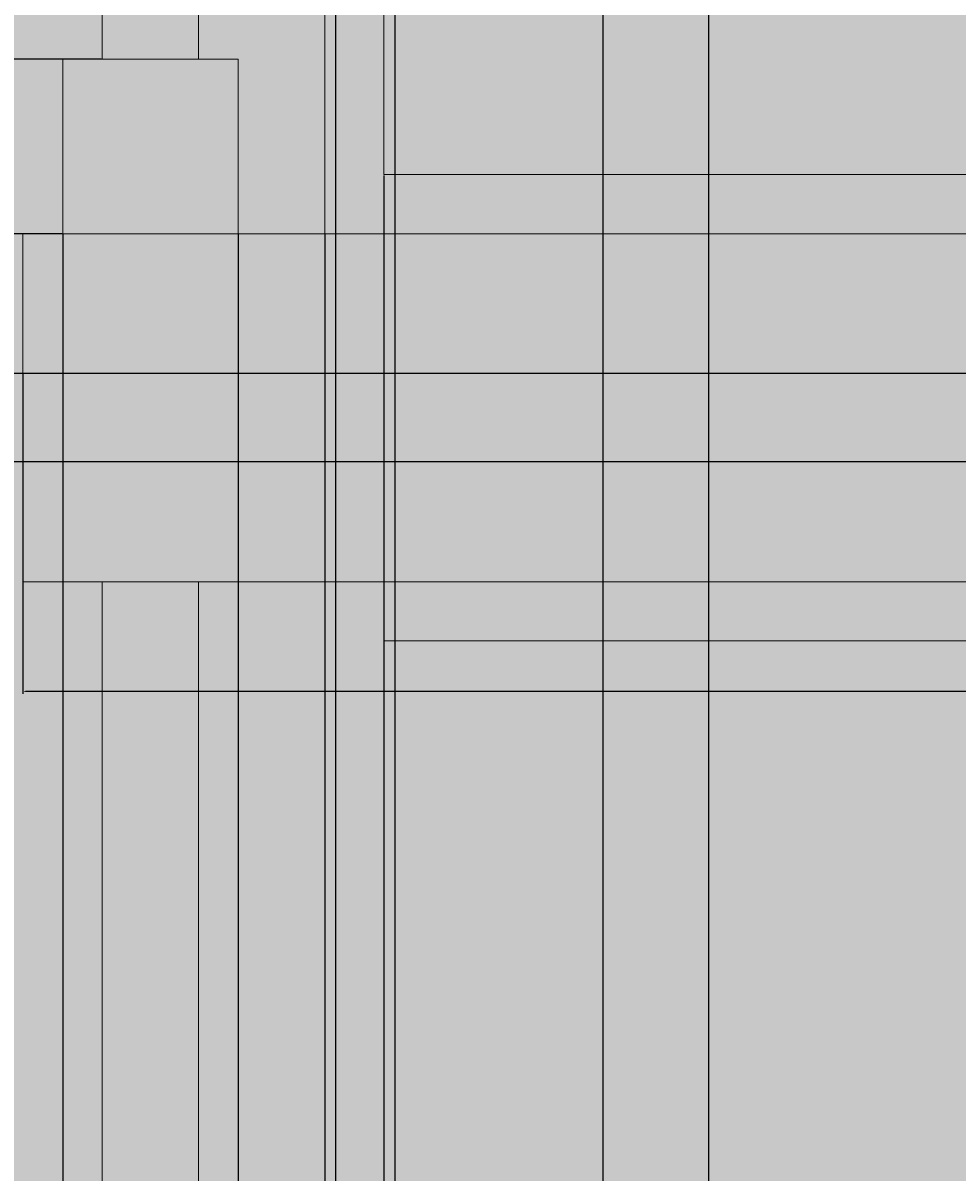
# Model space of a CAD drawing. Units: inches. Extents: x 3024 to 4744, y 1110 to 2100.
# Tile 20 of 29: x 3149 to 3212, y 1731 to 1809. Entities that reach past the tile are written whole.
import ezdxf

# ---------------------------------------------------------------- set-up
doc = ezdxf.new("R2010")
doc.units = ezdxf.units.IN
for name, color, linetype, lineweight in [('A-ANNO-DIMS', 2, 'Continuous', 18), ('A-ELEV', 7, 'Continuous', 25), ('A-ELEV-PATT', 252, 'Continuous', 13), ('A-GLAZ', 4, 'Continuous', 18)]:
    doc.layers.add(name, color=color, linetype=linetype, lineweight=lineweight)
doc.styles.get("Standard").update_dxf_attribs({"font": 'arial.ttf'})
doc.dimstyles.get("Standard").update_dxf_attribs({"dimtxt": 0.18, "dimasz": 0.18, "dimexe": 0.18, "dimexo": 0.0625, "dimgap": 0.09, "dimtad": 0, "dimtih": 1, "dimtoh": 1, "dimdec": 1, "dimzin": 0, "dimdsep": 46, "dimlunit": 3, "dimtxsty": 'Standard', "dimcen": 0.09, "dimadec": 0, "dimazin": 0, "dimtfac": 1, "dimtdec": 1, "dimtofl": 0, "dimtmove": 0, "dimatfit": 3, "dimfxl": 1, "dimtolj": 1, "dimtzin": 0, "dimarcsym": 0})

# ---------------------------------------------------------------- blocks, each defined once
blk = doc.blocks.new('WIN-BALCONY-A')
for p, q in [((3169.396, 1897.488), (3148.969, 1897.488)), ((3169.396, 1897.488), (3148.969, 1897.488)), ((3169.396, 1897.488), (3292.605, 1897.488)), ((3169.396, 1897.488), (3292.605, 1897.488)), ((3169.396, 1795.043), (3148.969, 1795.043)), ((3169.396, 1795.043), (3148.969, 1795.043)), ((3169.396, 1795.043), (3292.605, 1795.043)), ((3169.396, 1795.043), (3292.605, 1795.043))]:
    blk.add_line(p, q)
for points in [[(3148.969, 1897.488), (3148.969, 1905.611), (3292.605, 1905.611), (3292.605, 1897.488)], [(3148.969, 1897.488), (3148.969, 1905.611), (3292.605, 1905.611), (3292.605, 1897.488)], [(3292.605, 1795.043), (3292.605, 1785.611), (3148.969, 1785.611), (3148.969, 1795.043)], [(3292.605, 1795.043), (3292.605, 1785.611), (3148.969, 1785.611), (3148.969, 1795.043)]]:
    blk.add_lwpolyline(points)
for points in [[(3154.329, 1806.867), (3160.859, 1806.867), (3160.859, 1897.488), (3154.329, 1897.488)], [(3154.329, 1806.867), (3160.859, 1806.867), (3160.859, 1897.488), (3154.329, 1897.488)], [(3272.178, 1795.043), (3169.396, 1795.043), (3169.396, 1897.488), (3272.178, 1897.488)], [(3272.178, 1795.043), (3169.396, 1795.043), (3169.396, 1897.488), (3272.178, 1897.488)], [(3268.178, 1799.043), (3173.396, 1799.043), (3173.396, 1893.488), (3268.178, 1893.488)], [(3268.178, 1799.043), (3173.396, 1799.043), (3173.396, 1893.488), (3268.178, 1893.488)], [(3163.527, 1795.043), (3151.66, 1795.043), (3151.66, 1806.867), (3163.527, 1806.867)], [(3163.527, 1795.043), (3151.66, 1795.043), (3151.66, 1806.867), (3163.527, 1806.867)]]:
    blk.add_lwpolyline(points, close=True)
blk = doc.blocks.new('*D6')
at = {"layer": 'A-ANNO-DIMS', "color": 0, "lineweight": -2, "transparency": 16777216}
for p, q in [((3148.969, 1785.549), (3148.969, 1763.886)), ((3292.605, 1785.549), (3292.605, 1763.886)), ((3149.149, 1764.066), (3218.852, 1764.066)), ((3292.425, 1764.066), (3222.723, 1764.066))]:
    blk.add_line(p, q, dxfattribs=at)
at = {"layer": 'A-ANNO-DIMS', "color": 0, "transparency": 16777216}
for points in [[(3149.149, 1764.096), (3149.149, 1764.036), (3148.969, 1764.066)], [(3292.425, 1764.096), (3292.425, 1764.036), (3292.605, 1764.066)]]:
    blk.add_solid(points, dxfattribs=at)
at = {"layer": 'Defpoints', "color": 0, "transparency": 16777216}
for p in [(3148.969, 1785.611), (3292.605, 1785.611), (3292.605, 1764.066)]:
    blk.add_point(p, dxfattribs=at)
at = {"layer": 'A-ANNO-DIMS', "color": 0, "transparency": 16777216, "insert": (3220.787, 1764.066), "char_height": 0.18, "attachment_point": 5}
blk.add_mtext('\\A1;BALCONY WINDOW A 144 TYP.', dxfattribs=at)
blk = doc.blocks.new('*D64')
at = {"layer": 'A-ANNO-DIMS', "color": 0, "lineweight": -2, "transparency": 16777216}
for p, q in [((3069.794, 1241.497), (3069.794, 2100.438)), ((3741.151, 1241.497), (3741.151, 2100.438)), ((3069.974, 2100.258), (3405.078, 2100.258)), ((3740.971, 2100.258), (3405.866, 2100.258))]:
    blk.add_line(p, q, dxfattribs=at)
at = {"layer": 'A-ANNO-DIMS', "color": 0, "transparency": 16777216}
for points in [[(3069.974, 2100.288), (3069.974, 2100.228), (3069.794, 2100.258)], [(3740.971, 2100.288), (3740.971, 2100.228), (3741.151, 2100.258)]]:
    blk.add_solid(points, dxfattribs=at)
at = {"layer": 'Defpoints', "color": 0, "transparency": 16777216}
for p in [(3741.151, 2100.258), (3069.794, 1241.434), (3741.151, 1241.434)]:
    blk.add_point(p, dxfattribs=at)
at = {"layer": 'A-ANNO-DIMS', "color": 0, "transparency": 16777216, "insert": (3405.472, 2100.258), "char_height": 0.18, "attachment_point": 5}
blk.add_mtext('\\A1;671.4', dxfattribs=at)
blk = doc.blocks.new('*D89')
at = {"layer": 'A-ANNO-DIMS', "color": 0, "lineweight": -2, "transparency": 16777216}
for p, q in [((3151.66, 1794.981), (3151.66, 1109.931)), ((3163.527, 1794.981), (3163.527, 1109.931)), ((3151.84, 1110.111), (3157.139, 1110.111)), ((3163.347, 1110.111), (3158.049, 1110.111))]:
    blk.add_line(p, q, dxfattribs=at)
at = {"layer": 'A-ANNO-DIMS', "color": 0, "transparency": 16777216}
for points in [[(3151.84, 1110.141), (3151.84, 1110.081), (3151.66, 1110.111)], [(3163.347, 1110.141), (3163.347, 1110.081), (3163.527, 1110.111)]]:
    blk.add_solid(points, dxfattribs=at)
at = {"layer": 'Defpoints', "color": 0, "transparency": 16777216}
for p in [(3151.66, 1795.043), (3163.527, 1795.043), (3163.527, 1110.111)]:
    blk.add_point(p, dxfattribs=at)
at = {"layer": 'A-ANNO-DIMS', "color": 0, "transparency": 16777216, "insert": (3157.594, 1110.111), "char_height": 0.18, "attachment_point": 5}
blk.add_mtext('\\A1;11.866', dxfattribs=at)
blk = doc.blocks.new('*D90')
at = {"layer": 'A-ANNO-DIMS', "color": 0, "lineweight": -2, "transparency": 16777216}
for p, q in [((3173.396, 1798.981), (3173.396, 1109.931)), ((3169.396, 1794.981), (3169.396, 1109.931)), ((3169.576, 1110.111), (3171.069, 1110.111)), ((3173.216, 1110.111), (3171.723, 1110.111))]:
    blk.add_line(p, q, dxfattribs=at)
at = {"layer": 'A-ANNO-DIMS', "color": 0, "transparency": 16777216}
for points in [[(3169.576, 1110.141), (3169.576, 1110.081), (3169.396, 1110.111)], [(3173.216, 1110.141), (3173.216, 1110.081), (3173.396, 1110.111)]]:
    blk.add_solid(points, dxfattribs=at)
at = {"layer": 'Defpoints', "color": 0, "transparency": 16777216}
for p in [(3173.396, 1799.043), (3169.396, 1795.043), (3173.396, 1110.111)]:
    blk.add_point(p, dxfattribs=at)
at = {"layer": 'A-ANNO-DIMS', "color": 0, "transparency": 16777216, "insert": (3171.396, 1110.111), "char_height": 0.18, "attachment_point": 5}
blk.add_mtext('\\A1;4.00', dxfattribs=at)
blk = doc.blocks.new('*D91')
at = {"layer": 'A-ANNO-DIMS', "color": 0, "lineweight": -2, "transparency": 16777216}
for p, q in [((3173.396, 1798.981), (3173.396, 1109.931)), ((3220.05, 1798.981), (3220.05, 1109.931)), ((3173.576, 1110.111), (3196.325, 1110.111)), ((3219.87, 1110.111), (3197.121, 1110.111))]:
    blk.add_line(p, q, dxfattribs=at)
at = {"layer": 'A-ANNO-DIMS', "color": 0, "transparency": 16777216}
for points in [[(3173.576, 1110.141), (3173.576, 1110.081), (3173.396, 1110.111)], [(3219.87, 1110.141), (3219.87, 1110.081), (3220.05, 1110.111)]]:
    blk.add_solid(points, dxfattribs=at)
at = {"layer": 'Defpoints', "color": 0, "transparency": 16777216}
for p in [(3173.396, 1799.043), (3220.05, 1799.043), (3220.05, 1110.111)]:
    blk.add_point(p, dxfattribs=at)
at = {"layer": 'A-ANNO-DIMS', "color": 0, "transparency": 16777216, "insert": (3196.723, 1110.111), "char_height": 0.18, "attachment_point": 5}
blk.add_mtext('\\A1;46.65', dxfattribs=at)
blk = doc.blocks.new('*D97')
at = {"layer": 'A-ANNO-DIMS', "color": 0, "lineweight": -2, "transparency": 16777216}
for p, q in [((3151.598, 1806.867), (3024.114, 1806.867)), ((3024.294, 1806.687), (3024.294, 1801.137)), ((3024.294, 1795.223), (3024.294, 1800.773)), ((3151.598, 1795.043), (3024.114, 1795.043))]:
    blk.add_line(p, q, dxfattribs=at)
at = {"layer": 'A-ANNO-DIMS', "color": 0, "transparency": 16777216}
for points in [[(3024.264, 1806.687), (3024.324, 1806.687), (3024.294, 1806.867)], [(3024.264, 1795.223), (3024.324, 1795.223), (3024.294, 1795.043)]]:
    blk.add_solid(points, dxfattribs=at)
at = {"layer": 'Defpoints', "color": 0, "transparency": 16777216}
for p in [(3024.294, 1806.867), (3151.66, 1806.867), (3151.66, 1795.043)]:
    blk.add_point(p, dxfattribs=at)
at = {"layer": 'A-ANNO-DIMS', "color": 0, "transparency": 16777216, "insert": (3024.294, 1800.955), "char_height": 0.18, "attachment_point": 5}
blk.add_mtext('\\A1;11.824', dxfattribs=at)
blk = doc.blocks.new('*D98')
at = {"layer": 'A-ANNO-DIMS', "color": 0, "lineweight": -2, "transparency": 16777216}
for p, q in [((3154.266, 1897.488), (3024.114, 1897.488)), ((3024.294, 1897.308), (3024.294, 1852.36)), ((3024.294, 1807.047), (3024.294, 1851.996)), ((3154.266, 1806.867), (3024.114, 1806.867))]:
    blk.add_line(p, q, dxfattribs=at)
at = {"layer": 'A-ANNO-DIMS', "color": 0, "transparency": 16777216}
for points in [[(3024.264, 1897.308), (3024.324, 1897.308), (3024.294, 1897.488)], [(3024.264, 1807.047), (3024.324, 1807.047), (3024.294, 1806.867)]]:
    blk.add_solid(points, dxfattribs=at)
at = {"layer": 'Defpoints', "color": 0, "transparency": 16777216}
for p in [(3024.294, 1897.488), (3154.329, 1897.488), (3154.329, 1806.867)]:
    blk.add_point(p, dxfattribs=at)
at = {"layer": 'A-ANNO-DIMS', "color": 0, "transparency": 16777216, "insert": (3024.294, 1852.178), "char_height": 0.18, "attachment_point": 5}
blk.add_mtext('\\A1;90.62', dxfattribs=at)
blk = doc.blocks.new('*D106')
at = {"layer": 'A-ANNO-DIMS', "color": 0, "lineweight": -2, "transparency": 16777216}
for p, q in [((3170.161, 1275.674), (3170.161, 2100.438)), ((3174.161, 1271.674), (3174.161, 2100.438)), ((3170.341, 2100.258), (3171.834, 2100.258)), ((3173.981, 2100.258), (3172.488, 2100.258))]:
    blk.add_line(p, q, dxfattribs=at)
at = {"layer": 'A-ANNO-DIMS', "color": 0, "transparency": 16777216}
for points in [[(3170.341, 2100.288), (3170.341, 2100.228), (3170.161, 2100.258)], [(3173.981, 2100.288), (3173.981, 2100.228), (3174.161, 2100.258)]]:
    blk.add_solid(points, dxfattribs=at)
at = {"layer": 'Defpoints', "color": 0, "transparency": 16777216}
for p in [(3174.161, 2100.258), (3170.161, 1275.611), (3174.161, 1271.611)]:
    blk.add_point(p, dxfattribs=at)
at = {"layer": 'A-ANNO-DIMS', "color": 0, "transparency": 16777216, "insert": (3172.161, 2100.258), "char_height": 0.18, "attachment_point": 5}
blk.add_mtext('\\A1;4.00', dxfattribs=at)
blk = doc.blocks.new('*D107')
at = {"layer": 'A-ANNO-DIMS', "color": 0, "lineweight": -2, "transparency": 16777216}
for p, q in [((3174.161, 1271.674), (3174.161, 2100.438)), ((3270.388, 1271.674), (3270.388, 2100.438)), ((3174.341, 2100.258), (3221.881, 2100.258)), ((3270.208, 2100.258), (3222.668, 2100.258))]:
    blk.add_line(p, q, dxfattribs=at)
at = {"layer": 'A-ANNO-DIMS', "color": 0, "transparency": 16777216}
for points in [[(3174.341, 2100.288), (3174.341, 2100.228), (3174.161, 2100.258)], [(3270.208, 2100.288), (3270.208, 2100.228), (3270.388, 2100.258)]]:
    blk.add_solid(points, dxfattribs=at)
at = {"layer": 'Defpoints', "color": 0, "transparency": 16777216}
for p in [(3270.388, 2100.258), (3174.161, 1271.611), (3270.388, 1271.611)]:
    blk.add_point(p, dxfattribs=at)
at = {"layer": 'A-ANNO-DIMS', "color": 0, "transparency": 16777216, "insert": (3222.274, 2100.258), "char_height": 0.18, "attachment_point": 5}
blk.add_mtext('\\A1;96.23', dxfattribs=at)
blk = doc.blocks.new('*D124')
at = {"layer": 'A-ANNO-DIMS', "color": 0, "lineweight": -2, "transparency": 16777216}
for p, q in [((3174.161, 1271.674), (3174.161, 2100.438)), ((3188.259, 1256.29), (3188.259, 2100.438)), ((3174.341, 2100.258), (3180.754, 2100.258)), ((3188.079, 2100.258), (3181.665, 2100.258))]:
    blk.add_line(p, q, dxfattribs=at)
at = {"layer": 'A-ANNO-DIMS', "color": 0, "transparency": 16777216}
for points in [[(3174.341, 2100.288), (3174.341, 2100.228), (3174.161, 2100.258)], [(3188.079, 2100.288), (3188.079, 2100.228), (3188.259, 2100.258)]]:
    blk.add_solid(points, dxfattribs=at)
at = {"layer": 'Defpoints', "color": 0, "transparency": 16777216}
for p in [(3188.259, 2100.258), (3174.161, 1271.611), (3188.259, 1256.228)]:
    blk.add_point(p, dxfattribs=at)
at = {"layer": 'A-ANNO-DIMS', "color": 0, "transparency": 16777216, "insert": (3181.21, 2100.258), "char_height": 0.18, "attachment_point": 5}
blk.add_mtext('\\A1;14.098', dxfattribs=at)
blk = doc.blocks.new('*D125')
at = {"layer": 'A-ANNO-DIMS', "color": 0, "lineweight": -2, "transparency": 16777216}
for p, q in [((3188.259, 1256.29), (3188.259, 2100.438)), ((3195.405, 1256.29), (3195.405, 2100.438)), ((3188.439, 2100.258), (3191.439, 2100.258)), ((3195.225, 2100.258), (3192.225, 2100.258))]:
    blk.add_line(p, q, dxfattribs=at)
at = {"layer": 'A-ANNO-DIMS', "color": 0, "transparency": 16777216}
for points in [[(3188.439, 2100.288), (3188.439, 2100.228), (3188.259, 2100.258)], [(3195.225, 2100.288), (3195.225, 2100.228), (3195.405, 2100.258)]]:
    blk.add_solid(points, dxfattribs=at)
at = {"layer": 'Defpoints', "color": 0, "transparency": 16777216}
for p in [(3195.405, 2100.258), (3188.259, 1256.228), (3195.405, 1256.228)]:
    blk.add_point(p, dxfattribs=at)
at = {"layer": 'A-ANNO-DIMS', "color": 0, "transparency": 16777216, "insert": (3191.832, 2100.258), "char_height": 0.18, "attachment_point": 5}
blk.add_mtext('\\A1;7.147', dxfattribs=at)

msp = doc.modelspace()

# ---------------------------------------------------------------- hatches: boundary and pattern name
at = {"layer": 'A-ELEV-PATT'}
h = msp.add_hatch(color=256, dxfattribs=at)
h.dxf.hatch_style = 1
h.paths.add_polyline_path([(3491.8271, 2054.7584), (3320.5658, 2054.7584), (3320.5658, 2043.5286), (3491.8271, 2043.5286)])
h.paths.add_polyline_path([(3292.6051, 1905.6112), (3148.9694, 1905.6112), (3148.9694, 1897.4879), (3169.3964, 1897.4879), (3292.6051, 1897.4879)])
h.paths.add_polyline_path([(3292.6051, 1795.0431), (3169.3964, 1795.0431), (3148.9694, 1795.0431), (3148.9694, 1785.6112), (3292.6051, 1785.6112)])
h.paths.add_polyline_path([(3292.6051, 1779.6112), (3148.9694, 1779.6112), (3148.9694, 1771.4879), (3169.3964, 1771.4879), (3292.6051, 1771.4879)])
h.paths.add_polyline_path([(3292.6051, 1669.0431), (3169.3964, 1669.0431), (3148.9694, 1669.0431), (3148.9694, 1659.6112), (3292.6051, 1659.6112)])
h.paths.add_polyline_path([(3292.6051, 1653.6112), (3148.9694, 1653.6112), (3148.9694, 1645.4879), (3169.3964, 1645.4879), (3292.6051, 1645.4879)])
h.paths.add_polyline_path([(3292.6051, 1543.0431), (3169.3964, 1543.0431), (3148.9694, 1543.0431), (3148.9694, 1533.6112), (3292.6051, 1533.6112)])
h.paths.add_polyline_path([(3292.6051, 1527.6112), (3148.9694, 1527.6112), (3148.9694, 1519.4879), (3169.3964, 1519.4879), (3292.6051, 1519.4879)])
h.paths.add_polyline_path([(3292.6051, 1401.6112), (3148.9694, 1401.6112), (3148.9694, 1393.4879), (3169.3964, 1393.4879), (3292.6051, 1393.4879)])
h.paths.add_polyline_path([(3292.6051, 1417.0431), (3169.3964, 1417.0431), (3148.9694, 1417.0431), (3148.9694, 1407.6112), (3292.6051, 1407.6112)])
h.paths.add_polyline_path([(3292.6051, 1291.0431), (3169.3964, 1291.0431), (3148.9694, 1291.0431), (3148.9694, 1281.6112), (3292.6051, 1281.6112)])
h.paths.add_polyline_path([(3654.037, 1165.0431), (3530.8283, 1165.0431), (3510.4013, 1165.0431), (3510.4013, 1155.6112), (3654.037, 1155.6112)])
h.paths.add_polyline_path([(3654.037, 1275.6112), (3510.4013, 1275.6112), (3510.4013, 1267.4879), (3530.8283, 1267.4879), (3654.037, 1267.4879)])
h.paths.add_polyline_path([(3654.037, 1291.0431), (3530.8283, 1291.0431), (3510.4013, 1291.0431), (3510.4013, 1281.6112), (3654.037, 1281.6112)])
h.paths.add_polyline_path([(3654.037, 1417.0431), (3530.8283, 1417.0431), (3510.4013, 1417.0431), (3510.4013, 1407.6112), (3654.037, 1407.6112)])
h.paths.add_polyline_path([(3654.037, 1401.6112), (3510.4013, 1401.6112), (3510.4013, 1393.4879), (3530.8283, 1393.4879), (3654.037, 1393.4879)])
h.paths.add_polyline_path([(3654.037, 1543.0431), (3530.8283, 1543.0431), (3510.4013, 1543.0431), (3510.4013, 1533.6112), (3654.037, 1533.6112)])
h.paths.add_polyline_path([(3654.037, 1527.6112), (3510.4013, 1527.6112), (3510.4013, 1519.4879), (3530.8283, 1519.4879), (3654.037, 1519.4879)])
h.paths.add_polyline_path([(3654.037, 1653.6112), (3510.4013, 1653.6112), (3510.4013, 1645.4879), (3530.8283, 1645.4879), (3654.037, 1645.4879)])
h.paths.add_polyline_path([(3654.037, 1669.0431), (3530.8283, 1669.0431), (3510.4013, 1669.0431), (3510.4013, 1659.6112), (3654.037, 1659.6112)])
h.paths.add_polyline_path([(3654.037, 1779.6112), (3510.4013, 1779.6112), (3510.4013, 1771.4879), (3530.8283, 1771.4879), (3654.037, 1771.4879)])
h.paths.add_polyline_path([(3654.037, 1795.0431), (3530.8283, 1795.0431), (3510.4013, 1795.0431), (3510.4013, 1785.6112), (3654.037, 1785.6112)])
h.paths.add_polyline_path([(3654.037, 1905.6112), (3510.4013, 1905.6112), (3510.4013, 1897.4879), (3530.8283, 1897.4879), (3654.037, 1897.4879)])
h = msp.add_hatch(color=256, dxfattribs=at)
h.dxf.hatch_style = 1
h.paths.add_polyline_path([(3329.7033, 1407.6112), (3105.4722, 1407.6112), (3105.4722, 1401.6112), (3329.7033, 1401.6112)])
h.paths.add_polyline_path([(3329.7033, 1281.6112), (3105.4722, 1281.6112), (3105.4722, 1275.6112), (3112.3838, 1275.6112), (3329.7033, 1275.6112)])
h.paths.add_polyline_path([(3329.7033, 1533.6112), (3105.4722, 1533.6112), (3105.4722, 1527.6112), (3329.7033, 1527.6112)])
h.paths.add_polyline_path([(3329.7033, 1659.6112), (3105.4722, 1659.6112), (3105.4722, 1653.6112), (3329.7033, 1653.6112)])
h.paths.add_polyline_path([(3329.7033, 1785.6112), (3105.4722, 1785.6112), (3105.4722, 1779.6112), (3329.7033, 1779.6112)])
h.paths.add_polyline_path([(3329.7033, 1911.6112), (3105.4722, 1911.6112), (3095.7158, 1911.6112), (3095.7158, 1905.6112), (3329.7033, 1905.6112)])
h.paths.add_polyline_path([(3715.2286, 1911.6112), (3705.4722, 1911.6112), (3705.4722, 1905.6112), (3715.2286, 1905.6112)])
h.paths.add_polyline_path([(3688.5588, 1911.6112), (3481.2411, 1911.6112), (3481.2411, 1905.6112), (3688.5588, 1905.6112)])
h = msp.add_hatch(color=256, dxfattribs=at)
h.dxf.hatch_style = 1
h.paths.add_polyline_path([(3154.3287, 1897.4879), (3148.9694, 1897.4879), (3148.9694, 1905.6112), (3105.4722, 1905.6112), (3105.4722, 1785.6112), (3148.9694, 1785.6112), (3148.9694, 1795.0431), (3151.6604, 1795.0431), (3151.6604, 1806.8674), (3154.3287, 1806.8674)])
h.paths.add_polyline_path([(3329.7033, 1905.6112), (3292.6051, 1905.6112), (3292.6051, 1897.4879), (3287.2458, 1897.4879), (3287.2458, 1806.8674), (3288.3759, 1806.8674), (3288.3759, 1795.0431), (3292.6051, 1795.0431), (3292.6051, 1785.6112), (3329.7033, 1785.6112)])
h.paths.add_polyline_path([(3154.3287, 1771.4879), (3148.9694, 1771.4879), (3148.9694, 1779.6112), (3105.4722, 1779.6112), (3105.4722, 1659.6112), (3148.9694, 1659.6112), (3148.9694, 1669.0431), (3151.6604, 1669.0431), (3151.6604, 1680.8674), (3154.3287, 1680.8674)])
h.paths.add_polyline_path([(3329.7033, 1779.6112), (3292.6051, 1779.6112), (3292.6051, 1771.4879), (3287.2458, 1771.4879), (3287.2458, 1680.8674), (3288.3759, 1680.8674), (3288.3759, 1669.0431), (3292.6051, 1669.0431), (3292.6051, 1659.6112), (3329.7033, 1659.6112)])
h.paths.add_polyline_path([(3154.3287, 1645.4879), (3148.9694, 1645.4879), (3148.9694, 1653.6112), (3105.4722, 1653.6112), (3105.4722, 1533.6112), (3148.9694, 1533.6112), (3148.9694, 1543.0431), (3151.6604, 1543.0431), (3151.6604, 1554.8674), (3154.3287, 1554.8674)])
h.paths.add_polyline_path([(3329.7033, 1653.6112), (3292.6051, 1653.6112), (3292.6051, 1645.4879), (3287.2458, 1645.4879), (3287.2458, 1554.8674), (3288.3759, 1554.8674), (3288.3759, 1543.0431), (3292.6051, 1543.0431), (3292.6051, 1533.6112), (3329.7033, 1533.6112)])
h.paths.add_polyline_path([(3329.7033, 1527.6112), (3292.6051, 1527.6112), (3292.6051, 1519.4879), (3287.2458, 1519.4879), (3287.2458, 1428.8674), (3288.3759, 1428.8674), (3288.3759, 1417.0431), (3292.6051, 1417.0431), (3292.6051, 1407.6112), (3329.7033, 1407.6112)])
h.paths.add_polyline_path([(3329.7033, 1401.6112), (3292.6051, 1401.6112), (3292.6051, 1393.4879), (3287.2458, 1393.4879), (3287.2458, 1302.8674), (3288.3759, 1302.8674), (3288.3759, 1291.0431), (3292.6051, 1291.0431), (3292.6051, 1281.6112), (3329.7033, 1281.6112)])
h.paths.add_polyline_path([(3154.3287, 1393.4879), (3148.9694, 1393.4879), (3148.9694, 1401.6112), (3105.4722, 1401.6112), (3105.4722, 1281.6112), (3148.9694, 1281.6112), (3148.9694, 1291.0431), (3151.6604, 1291.0431), (3151.6604, 1302.8674), (3154.3287, 1302.8674)])
h.paths.add_polyline_path([(3154.3287, 1519.4879), (3148.9694, 1519.4879), (3148.9694, 1527.6112), (3105.4722, 1527.6112), (3105.4722, 1407.6112), (3148.9694, 1407.6112), (3148.9694, 1417.0431), (3151.6604, 1417.0431), (3151.6604, 1428.8674), (3154.3287, 1428.8674)])
h.paths.add_polyline_path([(3515.7606, 1897.4879), (3510.4013, 1897.4879), (3510.4013, 1905.6112), (3481.2411, 1905.6112), (3481.2411, 1785.6112), (3510.4013, 1785.6112), (3510.4013, 1795.0431), (3513.0923, 1795.0431), (3513.0923, 1806.8674), (3515.7606, 1806.8674)])
h.paths.add_polyline_path([(3688.5588, 1905.6112), (3654.037, 1905.6112), (3654.037, 1897.4879), (3648.6777, 1897.4879), (3648.6777, 1806.8674), (3649.8078, 1806.8674), (3649.8078, 1795.0431), (3654.037, 1795.0431), (3654.037, 1785.6112), (3688.5588, 1785.6112)])
h.paths.add_polyline_path([(3515.7606, 1771.4879), (3510.4013, 1771.4879), (3510.4013, 1779.6112), (3481.2411, 1779.6112), (3481.2411, 1659.6112), (3510.4013, 1659.6112), (3510.4013, 1669.0431), (3513.0923, 1669.0431), (3513.0923, 1680.8674), (3515.7606, 1680.8674)])
h.paths.add_polyline_path([(3688.5588, 1779.6112), (3654.037, 1779.6112), (3654.037, 1771.4879), (3648.6777, 1771.4879), (3648.6777, 1680.8674), (3649.8078, 1680.8674), (3649.8078, 1669.0431), (3654.037, 1669.0431), (3654.037, 1659.6112), (3688.5588, 1659.6112)])
h.paths.add_polyline_path([(3515.7606, 1645.4879), (3510.4013, 1645.4879), (3510.4013, 1653.6112), (3481.2411, 1653.6112), (3481.2411, 1533.6112), (3510.4013, 1533.6112), (3510.4013, 1543.0431), (3513.0923, 1543.0431), (3513.0923, 1554.8674), (3515.7606, 1554.8674)])
h.paths.add_polyline_path([(3688.5588, 1653.6112), (3654.037, 1653.6112), (3654.037, 1645.4879), (3648.6777, 1645.4879), (3648.6777, 1554.8674), (3649.8078, 1554.8674), (3649.8078, 1543.0431), (3654.037, 1543.0431), (3654.037, 1533.6112), (3688.5588, 1533.6112)])
h.paths.add_polyline_path([(3515.7606, 1519.4879), (3510.4013, 1519.4879), (3510.4013, 1527.6112), (3481.2411, 1527.6112), (3481.2411, 1407.6112), (3510.4013, 1407.6112), (3510.4013, 1417.0431), (3513.0923, 1417.0431), (3513.0923, 1428.8674), (3515.7606, 1428.8674)])
h.paths.add_polyline_path([(3688.5588, 1527.6112), (3654.037, 1527.6112), (3654.037, 1519.4879), (3648.6777, 1519.4879), (3648.6777, 1428.8674), (3649.8078, 1428.8674), (3649.8078, 1417.0431), (3654.037, 1417.0431), (3654.037, 1407.6112), (3688.5588, 1407.6112)])
h.paths.add_polyline_path([(3515.7606, 1393.4879), (3510.4013, 1393.4879), (3510.4013, 1401.6112), (3481.2411, 1401.6112), (3481.2411, 1281.6112), (3510.4013, 1281.6112), (3510.4013, 1291.0431), (3513.0923, 1291.0431), (3513.0923, 1302.8674), (3515.7606, 1302.8674)])
h.paths.add_polyline_path([(3688.5588, 1401.6112), (3654.037, 1401.6112), (3654.037, 1393.4879), (3648.6777, 1393.4879), (3648.6777, 1302.8674), (3649.8078, 1302.8674), (3649.8078, 1291.0431), (3654.037, 1291.0431), (3654.037, 1281.6112), (3688.5588, 1281.6112)])
h.paths.add_polyline_path([(3515.7606, 1267.4879), (3510.4013, 1267.4879), (3510.4013, 1275.6112), (3481.2411, 1275.6112), (3481.2411, 1155.6112), (3510.4013, 1155.6112), (3510.4013, 1165.0431), (3513.0923, 1165.0431), (3513.0923, 1176.8674), (3515.7606, 1176.8674)])
h.paths.add_polyline_path([(3688.5588, 1275.6112), (3654.037, 1275.6112), (3654.037, 1267.4879), (3648.6777, 1267.4879), (3648.6777, 1176.8674), (3649.8078, 1176.8674), (3649.8078, 1165.0431), (3654.037, 1165.0431), (3654.037, 1155.6112), (3688.5588, 1155.6112)])
h.paths.add_polyline_path([(3112.3838, 1275.6112), (3105.4722, 1275.6112), (3105.4722, 1171.0239), (3112.3838, 1171.0239)])
h = msp.add_hatch(color=256, dxfattribs=at)
h.dxf.hatch_style = 1
h.paths.add_polyline_path([(3160.8586, 1897.4879), (3154.3287, 1897.4879), (3154.3287, 1806.8674), (3160.8586, 1806.8674)])
h.paths.add_polyline_path([(3287.2458, 1897.4879), (3280.716, 1897.4879), (3280.716, 1806.8674), (3287.2458, 1806.8674)])
h.paths.add_polyline_path([(3160.8586, 1771.4879), (3154.3287, 1771.4879), (3154.3287, 1680.8674), (3160.8586, 1680.8674)])
h.paths.add_polyline_path([(3287.2458, 1771.4879), (3280.716, 1771.4879), (3280.716, 1680.8674), (3287.2458, 1680.8674)])
h.paths.add_polyline_path([(3160.8586, 1645.4879), (3154.3287, 1645.4879), (3154.3287, 1554.8674), (3160.8586, 1554.8674)])
h.paths.add_polyline_path([(3287.2458, 1645.4879), (3280.716, 1645.4879), (3280.716, 1554.8674), (3287.2458, 1554.8674)])
h.paths.add_polyline_path([(3160.8586, 1519.4879), (3154.3287, 1519.4879), (3154.3287, 1428.8674), (3160.8586, 1428.8674)])
h.paths.add_polyline_path([(3287.2458, 1519.4879), (3280.716, 1519.4879), (3280.716, 1428.8674), (3287.2458, 1428.8674)])
h.paths.add_polyline_path([(3160.8586, 1393.4879), (3154.3287, 1393.4879), (3154.3287, 1302.8674), (3160.8586, 1302.8674)])
h.paths.add_polyline_path([(3287.2458, 1393.4879), (3280.716, 1393.4879), (3280.716, 1302.8674), (3287.2458, 1302.8674)])
h.paths.add_polyline_path([(3648.6777, 1267.4879), (3642.1479, 1267.4879), (3642.1479, 1176.8674), (3648.6777, 1176.8674)])
h.paths.add_polyline_path([(3522.2905, 1267.4879), (3515.7606, 1267.4879), (3515.7606, 1176.8674), (3522.2905, 1176.8674)])
h.paths.add_polyline_path([(3522.2905, 1393.4879), (3515.7606, 1393.4879), (3515.7606, 1302.8674), (3522.2905, 1302.8674)])
h.paths.add_polyline_path([(3648.6777, 1393.4879), (3642.1479, 1393.4879), (3642.1479, 1302.8674), (3648.6777, 1302.8674)])
h.paths.add_polyline_path([(3522.2905, 1519.4879), (3515.7606, 1519.4879), (3515.7606, 1428.8674), (3522.2905, 1428.8674)])
h.paths.add_polyline_path([(3648.6777, 1519.4879), (3642.1479, 1519.4879), (3642.1479, 1428.8674), (3648.6777, 1428.8674)])
h.paths.add_polyline_path([(3522.2905, 1645.4879), (3515.7606, 1645.4879), (3515.7606, 1554.8674), (3522.2905, 1554.8674)])
h.paths.add_polyline_path([(3522.2905, 1771.4879), (3515.7606, 1771.4879), (3515.7606, 1680.8674), (3522.2905, 1680.8674)])
h.paths.add_polyline_path([(3648.6777, 1645.4879), (3642.1479, 1645.4879), (3642.1479, 1554.8674), (3648.6777, 1554.8674)])
h.paths.add_polyline_path([(3648.6777, 1771.4879), (3642.1479, 1771.4879), (3642.1479, 1680.8674), (3648.6777, 1680.8674)])
h.paths.add_polyline_path([(3648.6777, 1897.4879), (3642.1479, 1897.4879), (3642.1479, 1806.8674), (3648.6777, 1806.8674)])
h.paths.add_polyline_path([(3522.2905, 1897.4879), (3515.7606, 1897.4879), (3515.7606, 1806.8674), (3522.2905, 1806.8674)])
h = msp.add_hatch(color=256, dxfattribs=at)
h.dxf.hatch_style = 1
h.paths.add_polyline_path([(3169.3964, 1897.4879), (3160.8586, 1897.4879), (3160.8586, 1806.8674), (3163.5269, 1806.8674), (3163.5269, 1795.0431), (3169.3964, 1795.0431)])
h.paths.add_polyline_path([(3280.716, 1897.4879), (3272.1781, 1897.4879), (3272.1781, 1795.0431), (3276.5094, 1795.0431), (3276.5094, 1806.8674), (3280.716, 1806.8674)])
h.paths.add_polyline_path([(3280.716, 1771.4879), (3272.1781, 1771.4879), (3272.1781, 1669.0431), (3276.5094, 1669.0431), (3276.5094, 1680.8674), (3280.716, 1680.8674)])
h.paths.add_polyline_path([(3169.3964, 1771.4879), (3160.8586, 1771.4879), (3160.8586, 1680.8674), (3163.5269, 1680.8674), (3163.5269, 1669.0431), (3169.3964, 1669.0431)])
h.paths.add_polyline_path([(3169.3964, 1645.4879), (3160.8586, 1645.4879), (3160.8586, 1554.8674), (3163.5269, 1554.8674), (3163.5269, 1543.0431), (3169.3964, 1543.0431)])
h.paths.add_polyline_path([(3280.716, 1645.4879), (3272.1781, 1645.4879), (3272.1781, 1543.0431), (3276.5094, 1543.0431), (3276.5094, 1554.8674), (3280.716, 1554.8674)])
h.paths.add_polyline_path([(3169.3964, 1519.4879), (3160.8586, 1519.4879), (3160.8586, 1428.8674), (3163.5269, 1428.8674), (3163.5269, 1417.0431), (3169.3964, 1417.0431)])
h.paths.add_polyline_path([(3280.716, 1519.4879), (3272.1781, 1519.4879), (3272.1781, 1417.0431), (3276.5094, 1417.0431), (3276.5094, 1428.8674), (3280.716, 1428.8674)])
h.paths.add_polyline_path([(3169.3964, 1393.4879), (3160.8586, 1393.4879), (3160.8586, 1302.8674), (3163.5269, 1302.8674), (3163.5269, 1291.0431), (3169.3964, 1291.0431)])
h.paths.add_polyline_path([(3280.716, 1393.4879), (3272.1781, 1393.4879), (3272.1781, 1291.0431), (3276.5094, 1291.0431), (3276.5094, 1302.8674), (3280.716, 1302.8674)])
h.paths.add_polyline_path([(3642.1479, 1267.4879), (3633.61, 1267.4879), (3633.61, 1165.0431), (3637.9413, 1165.0431), (3637.9413, 1176.8674), (3642.1479, 1176.8674)])
h.paths.add_polyline_path([(3530.8283, 1267.4879), (3522.2905, 1267.4879), (3522.2905, 1176.8674), (3524.9588, 1176.8674), (3524.9588, 1165.0431), (3530.8283, 1165.0431)])
h.paths.add_polyline_path([(3642.1479, 1393.4879), (3633.61, 1393.4879), (3633.61, 1291.0431), (3637.9413, 1291.0431), (3637.9413, 1302.8674), (3642.1479, 1302.8674)])
h.paths.add_polyline_path([(3530.8283, 1393.4879), (3522.2905, 1393.4879), (3522.2905, 1302.8674), (3524.9588, 1302.8674), (3524.9588, 1291.0431), (3530.8283, 1291.0431)])
h.paths.add_polyline_path([(3530.8283, 1519.4879), (3522.2905, 1519.4879), (3522.2905, 1428.8674), (3524.9588, 1428.8674), (3524.9588, 1417.0431), (3530.8283, 1417.0431)])
h.paths.add_polyline_path([(3642.1479, 1519.4879), (3633.61, 1519.4879), (3633.61, 1417.0431), (3637.9413, 1417.0431), (3637.9413, 1428.8674), (3642.1479, 1428.8674)])
h.paths.add_polyline_path([(3530.8283, 1645.4879), (3522.2905, 1645.4879), (3522.2905, 1554.8674), (3524.9588, 1554.8674), (3524.9588, 1543.0431), (3530.8283, 1543.0431)])
h.paths.add_polyline_path([(3642.1479, 1645.4879), (3633.61, 1645.4879), (3633.61, 1543.0431), (3637.9413, 1543.0431), (3637.9413, 1554.8674), (3642.1479, 1554.8674)])
h.paths.add_polyline_path([(3642.1479, 1771.4879), (3633.61, 1771.4879), (3633.61, 1669.0431), (3637.9413, 1669.0431), (3637.9413, 1680.8674), (3642.1479, 1680.8674)])
h.paths.add_polyline_path([(3530.8283, 1771.4879), (3522.2905, 1771.4879), (3522.2905, 1680.8674), (3524.9588, 1680.8674), (3524.9588, 1669.0431), (3530.8283, 1669.0431)])
h.paths.add_polyline_path([(3530.8283, 1897.4879), (3522.2905, 1897.4879), (3522.2905, 1806.8674), (3524.9588, 1806.8674), (3524.9588, 1795.0431), (3530.8283, 1795.0431)])
h.paths.add_polyline_path([(3642.1479, 1897.4879), (3633.61, 1897.4879), (3633.61, 1795.0431), (3637.9413, 1795.0431), (3637.9413, 1806.8674), (3642.1479, 1806.8674)])
h = msp.add_hatch(color=256, dxfattribs=at)
h.dxf.hatch_style = 1
h.paths.add_polyline_path([(3221.5241, 1893.4879), (3220.0505, 1893.4879), (3220.0505, 1799.0431), (3221.5241, 1799.0431)], flags=0)
h.paths.add_polyline_path([(3272.1781, 1897.4879), (3169.3964, 1897.4879), (3169.3964, 1795.0431), (3272.1781, 1795.0431)])
h.paths.add_polyline_path([(3268.1781, 1893.4879), (3268.1781, 1799.0431), (3173.3964, 1799.0431), (3173.3964, 1893.4879)], flags=16)
h.paths.add_polyline_path([(3221.5241, 1893.4879), (3221.5241, 1799.0431), (3220.0505, 1799.0431), (3220.0505, 1893.4879)], flags=0)
h = msp.add_hatch(color=256, dxfattribs=at)
h.dxf.hatch_style = 1
h.paths.add_polyline_path([(3220.0505, 1893.4879), (3173.3964, 1893.4879), (3173.3964, 1799.0431), (3220.0505, 1799.0431)])
h.paths.add_polyline_path([(3268.1781, 1893.4879), (3221.5241, 1893.4879), (3221.5241, 1799.0431), (3268.1781, 1799.0431)])
h.paths.add_polyline_path([(3581.4824, 1893.4879), (3534.8283, 1893.4879), (3534.8283, 1799.0431), (3581.4824, 1799.0431)])
h.paths.add_polyline_path([(3629.61, 1893.4879), (3582.956, 1893.4879), (3582.956, 1799.0431), (3629.61, 1799.0431)])
h.paths.add_polyline_path([(3581.4824, 1767.4879), (3534.8283, 1767.4879), (3534.8283, 1673.0431), (3581.4824, 1673.0431)])
h.paths.add_polyline_path([(3629.61, 1767.4879), (3582.956, 1767.4879), (3582.956, 1673.0431), (3629.61, 1673.0431)])
h.paths.add_polyline_path([(3581.4824, 1641.4879), (3534.8283, 1641.4879), (3534.8283, 1547.0431), (3581.4824, 1547.0431)])
h.paths.add_polyline_path([(3629.61, 1641.4879), (3582.956, 1641.4879), (3582.956, 1547.0431), (3629.61, 1547.0431)])
h.paths.add_polyline_path([(3629.61, 1515.4879), (3582.956, 1515.4879), (3582.956, 1421.0431), (3629.61, 1421.0431)])
h.paths.add_polyline_path([(3581.4824, 1515.4879), (3534.8283, 1515.4879), (3534.8283, 1421.0431), (3581.4824, 1421.0431)])
h.paths.add_polyline_path([(3629.61, 1389.4879), (3582.956, 1389.4879), (3582.956, 1295.0431), (3629.61, 1295.0431)])
h.paths.add_polyline_path([(3581.4824, 1389.4879), (3534.8283, 1389.4879), (3534.8283, 1295.0431), (3581.4824, 1295.0431)])
h.paths.add_polyline_path([(3629.61, 1263.4879), (3582.956, 1263.4879), (3582.956, 1169.0431), (3629.61, 1169.0431)])
h.paths.add_polyline_path([(3581.4824, 1263.4879), (3534.8283, 1263.4879), (3534.8283, 1169.0431), (3581.4824, 1169.0431)])
h.paths.add_polyline_path([(3220.0505, 1389.4879), (3173.3964, 1389.4879), (3173.3964, 1295.0431), (3220.0505, 1295.0431)])
h.paths.add_polyline_path([(3268.1781, 1389.4879), (3221.5241, 1389.4879), (3221.5241, 1295.0431), (3268.1781, 1295.0431)])
h.paths.add_polyline_path([(3220.0505, 1515.4879), (3173.3964, 1515.4879), (3173.3964, 1421.0431), (3220.0505, 1421.0431)])
h.paths.add_polyline_path([(3268.1781, 1515.4879), (3221.5241, 1515.4879), (3221.5241, 1421.0431), (3268.1781, 1421.0431)])
h.paths.add_polyline_path([(3220.0505, 1767.4879), (3173.3964, 1767.4879), (3173.3964, 1673.0431), (3220.0505, 1673.0431)])
h.paths.add_polyline_path([(3268.1781, 1767.4879), (3221.5241, 1767.4879), (3221.5241, 1673.0431), (3268.1781, 1673.0431)])
h.paths.add_polyline_path([(3220.0505, 1641.4879), (3173.3964, 1641.4879), (3173.3964, 1547.0431), (3220.0505, 1547.0431)])
h.paths.add_polyline_path([(3268.1781, 1641.4879), (3221.5241, 1641.4879), (3221.5241, 1547.0431), (3268.1781, 1547.0431)])
h = msp.add_hatch(color=256, dxfattribs=at)
h.dxf.hatch_style = 1
h.paths.add_polyline_path([(3163.5269, 1302.8674), (3151.6604, 1302.8674), (3151.6604, 1291.0431), (3163.5269, 1291.0431)])
h.paths.add_polyline_path([(3288.3759, 1302.8674), (3276.5094, 1302.8674), (3276.5094, 1291.0431), (3288.3759, 1291.0431)])
h.paths.add_polyline_path([(3288.3759, 1428.8674), (3276.5094, 1428.8674), (3276.5094, 1417.0431), (3288.3759, 1417.0431)])
h.paths.add_polyline_path([(3163.5269, 1428.8674), (3151.6604, 1428.8674), (3151.6604, 1417.0431), (3163.5269, 1417.0431)])
h.paths.add_polyline_path([(3163.5269, 1554.8674), (3151.6604, 1554.8674), (3151.6604, 1543.0431), (3163.5269, 1543.0431)])
h.paths.add_polyline_path([(3288.3759, 1554.8674), (3276.5094, 1554.8674), (3276.5094, 1543.0431), (3288.3759, 1543.0431)])
h.paths.add_polyline_path([(3163.5269, 1680.8674), (3151.6604, 1680.8674), (3151.6604, 1669.0431), (3163.5269, 1669.0431)])
h.paths.add_polyline_path([(3288.3759, 1680.8674), (3276.5094, 1680.8674), (3276.5094, 1669.0431), (3288.3759, 1669.0431)])
h.paths.add_polyline_path([(3163.5269, 1806.8674), (3151.6604, 1806.8674), (3151.6604, 1795.0431), (3163.5269, 1795.0431)])
h.paths.add_polyline_path([(3288.3759, 1806.8674), (3276.5094, 1806.8674), (3276.5094, 1795.0431), (3288.3759, 1795.0431)])
h.paths.add_polyline_path([(3524.9588, 1806.8674), (3513.0923, 1806.8674), (3513.0923, 1795.0431), (3524.9588, 1795.0431)])
h.paths.add_polyline_path([(3649.8078, 1806.8674), (3637.9413, 1806.8674), (3637.9413, 1795.0431), (3649.8078, 1795.0431)])
h.paths.add_polyline_path([(3524.9588, 1680.8674), (3513.0923, 1680.8674), (3513.0923, 1669.0431), (3524.9588, 1669.0431)])
h.paths.add_polyline_path([(3649.8078, 1680.8674), (3637.9413, 1680.8674), (3637.9413, 1669.0431), (3649.8078, 1669.0431)])
h.paths.add_polyline_path([(3524.9588, 1554.8674), (3513.0923, 1554.8674), (3513.0923, 1543.0431), (3524.9588, 1543.0431)])
h.paths.add_polyline_path([(3649.8078, 1554.8674), (3637.9413, 1554.8674), (3637.9413, 1543.0431), (3649.8078, 1543.0431)])
h.paths.add_polyline_path([(3524.9588, 1428.8674), (3513.0923, 1428.8674), (3513.0923, 1417.0431), (3524.9588, 1417.0431)])
h.paths.add_polyline_path([(3649.8078, 1428.8674), (3637.9413, 1428.8674), (3637.9413, 1417.0431), (3649.8078, 1417.0431)])
h.paths.add_polyline_path([(3524.9588, 1302.8674), (3513.0923, 1302.8674), (3513.0923, 1291.0431), (3524.9588, 1291.0431)])
h.paths.add_polyline_path([(3649.8078, 1302.8674), (3637.9413, 1302.8674), (3637.9413, 1291.0431), (3649.8078, 1291.0431)])
h.paths.add_polyline_path([(3524.9588, 1176.8674), (3513.0923, 1176.8674), (3513.0923, 1165.0431), (3524.9588, 1165.0431)])
h.paths.add_polyline_path([(3649.8078, 1176.8674), (3637.9413, 1176.8674), (3637.9413, 1165.0431), (3649.8078, 1165.0431)])
h = msp.add_hatch(color=256, dxfattribs=at)
h.dxf.hatch_style = 1
h.paths.add_polyline_path([(3221.5241, 1767.4879), (3220.0505, 1767.4879), (3220.0505, 1673.0431), (3221.5241, 1673.0431)], flags=0)
h.paths.add_polyline_path([(3272.1781, 1771.4879), (3169.3964, 1771.4879), (3169.3964, 1669.0431), (3272.1781, 1669.0431)])
h.paths.add_polyline_path([(3268.1781, 1767.4879), (3268.1781, 1673.0431), (3173.3964, 1673.0431), (3173.3964, 1767.4879)], flags=16)
h.paths.add_polyline_path([(3221.5241, 1767.4879), (3221.5241, 1673.0431), (3220.0505, 1673.0431), (3220.0505, 1767.4879)], flags=0)

# ---------------------------------------------------------------- linework, layer by layer
at = {"layer": 'A-ELEV'}
for p, q in [((3105.4722, 1785.6112), (3329.7033, 1785.6112)), ((3105.4722, 1785.6112), (3329.7033, 1785.6112)), ((3329.7033, 1779.6112), (3105.4722, 1779.6112)), ((3329.7033, 1779.6112), (3105.4722, 1779.6112))]:
    msp.add_line(p, q, dxfattribs=at)

# ---------------------------------------------------------------- block references
at = {"layer": 'A-GLAZ'}
for p in [(0, 0), (0, -126)]:
    msp.add_blockref('WIN-BALCONY-A', p, dxfattribs=at)

# ---------------------------------------------------------------- dimensions: what is measured, and where the dimension line sits
at = {"layer": 'A-ANNO-DIMS'}
for base, p1, p2, override, picture, middle in [((3741.1507, 2100.2584), (3069.7937, 1241.4341), (3741.1507, 1241.4341), {"dimdec": 1, "dimlfac": 1, "dimrnd": 0, "dimzin": 0, "dimdsep": 46, "dimlunit": 2}, '*D64', (3405.4722, 2100.2584)), ((3174.1608, 2100.2584), (3170.1608, 1275.6112), (3174.1608, 1271.6112), {"dimdec": 2, "dimlfac": 1, "dimrnd": 0, "dimzin": 0, "dimdsep": 46, "dimlunit": 2}, '*D106', (3172.1608, 2100.2584)), ((3270.3877, 2100.2584), (3174.1608, 1271.6112), (3270.3877, 1271.6112), {"dimdec": 2, "dimlfac": 1, "dimrnd": 0, "dimzin": 0, "dimdsep": 46, "dimlunit": 2}, '*D107', (3222.2743, 2100.2584)), ((3188.2586, 2100.2584), (3174.1608, 1271.6112), (3188.2586, 1256.2276), {"dimdec": 3, "dimlfac": 1, "dimrnd": 0, "dimzin": 0, "dimdsep": 46, "dimlunit": 2}, '*D124', (3181.2097, 2100.2584)), ((3195.4053, 2100.2584), (3188.2586, 1256.2276), (3195.4053, 1256.2276), {"dimdec": 3, "dimlfac": 1, "dimrnd": 0, "dimzin": 0, "dimdsep": 46, "dimlunit": 2}, '*D125', (3191.832, 2100.2584)), ((3173.3964, 1110.1112), (3169.3964, 1795.0431), (3173.3964, 1799.0431), {"dimdec": 2, "dimlfac": 1, "dimrnd": 0, "dimzin": 0, "dimdsep": 46, "dimlunit": 2}, '*D90', (3171.3964, 1110.1112)), ((3220.0505, 1110.1112), (3173.3964, 1799.0431), (3220.0505, 1799.0431), {"dimdec": 2, "dimlfac": 1, "dimrnd": 0, "dimzin": 0, "dimdsep": 46, "dimlunit": 2}, '*D91', (3196.7234, 1110.1112)), ((3163.526875, 1110.111173), (3151.660378, 1795.043127), (3163.526875, 1795.043127), {"dimdec": 3, "dimlfac": 1, "dimrnd": 0, "dimzin": 0, "dimdsep": 46, "dimlunit": 2}, '*D89', (3157.593627, 1110.111173))]:
    dim = msp.add_linear_dim(base=base, p1=p1, p2=p2, dimstyle='Standard', override=override, dxfattribs=at)
    dim.commit()
    dim.dimension.update_dxf_attribs({"geometry": picture, "text_midpoint": middle})
for base, p1, p2, override, picture, middle in [((3024.2937, 1897.4879), (3154.3287, 1806.8674), (3154.3287, 1897.4879), {"dimdec": 2, "dimlfac": 1, "dimrnd": 0, "dimzin": 0, "dimdsep": 46, "dimlunit": 2}, '*D98', (3024.2937, 1852.1776)), ((3024.2937, 1806.8674), (3151.6604, 1795.0431), (3151.6604, 1806.8674), {"dimdec": 3, "dimlfac": 1, "dimrnd": 0, "dimzin": 0, "dimdsep": 46, "dimlunit": 2}, '*D97', (3024.2937, 1800.9553))]:
    dim = msp.add_linear_dim(base=base, p1=p1, p2=p2, angle=90, dimstyle='Standard', override=override, dxfattribs=at)
    dim.commit()
    dim.dimension.update_dxf_attribs({"geometry": picture, "text_midpoint": middle})
dim = msp.add_linear_dim(base=(3292.6051, 1764.0658), p1=(3148.9694, 1785.6112), p2=(3292.6051, 1785.6112), text='BALCONY WINDOW A <> TYP.', dimstyle='Standard', override={"dimdec": 0, "dimrnd": 0, "dimzin": 0, "dimlunit": 2}, dxfattribs=at)
dim.commit()
dim.dimension.update_dxf_attribs({"geometry": '*D6', "text_midpoint": (3220.7873, 1764.0658)})

doc.saveas('drawing.dxf')
